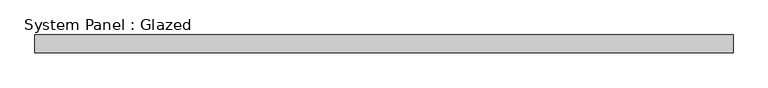
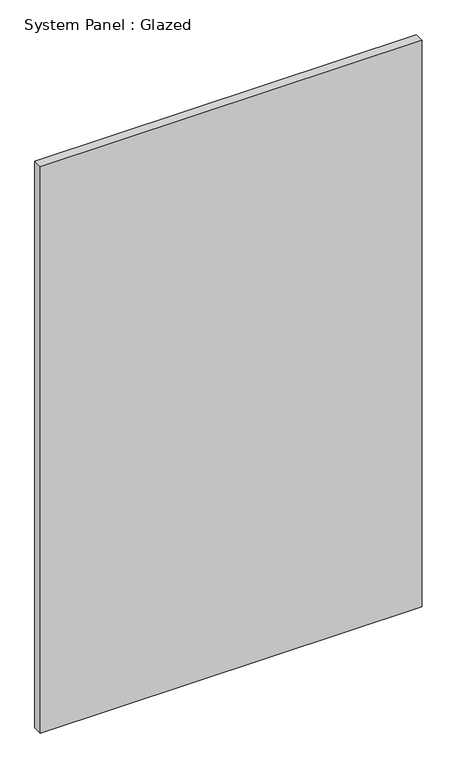
"""IFC4 building model written with IfcOpenShell, lengths in millimetres: plate geometry, System Panel : Glazed."""

from ifc_helpers import new_model, si_unit, origin, origin_with_axes, place, context, project, spatial, polyline, outline, extrude, source, transform, mapped, element, save


def system_panel_glazed_a32de224(model_context):
    return source(origin(), model_context, "Body", "SweptSolid", [
        extrude(outline(polyline([(501.65, 19.05), (-501.65, 19.05), (-501.65, 44.45), (501.65, 44.45), (501.65, 19.05)])), origin_with_axes(), (0.0, 0.0, 1.0), 1573.436135),
    ])


if __name__ == "__main__":
    model = new_model("IFC4")
    model_context = context("Model", 3, world=origin())
    ifc_project = project(units=[si_unit("LENGTHUNIT", "METRE", prefix="MILLI")], contexts=[model_context])
    site = spatial("IfcSite", under=ifc_project)
    building = spatial("IfcBuilding", under=site)
    placement = place(None, origin())
    system_panel_glazed_shape = system_panel_glazed_a32de224(model_context)
    element("IfcPlate", 1, ObjectType="System Panel : Glazed", at=placement, inside=building, context=model_context, shape_type="MappedRepresentation", body=[
        mapped(system_panel_glazed_shape, transform((0.0, 0.0, 0.0), x_axis=(1.0, 0.0, 0.0), y_axis=(0.0, 1.0, 0.0), z_axis=(0.0, 0.0, 1.0))),
    ])
    save(model, "model.ifc")

# Revit data of these elements
# Type "System Panel : Glazed"
#   Construction Type Id = "GSP4R"
#   Analytic Construction = "1/8 in Pilkington single glazing"
#   Visual Light Transmittance = 0.9
#   Solar Heat Gain Coefficient = 0.86
#   Heat Transfer Coefficient (U) = 1.18115 BTU/(h·ft²·°F)
#   Define Thermal Properties by = 1
# Element 1 (IfcPlate, "System Panel : Glazed")
#   Materials on its faces: "Glass"
# Materials
#   "Glass": class "Glass", colour RGB 0 128 192, transparency 0.75, Description = "Soda Lime Glass", Cost = 0
